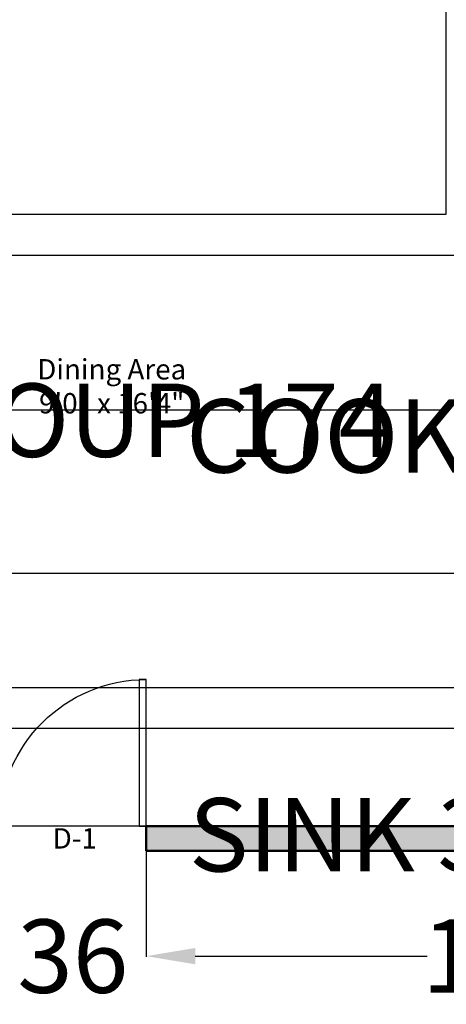
# Model space of a CAD drawing. Units: inches. Extents: x -478 to 256, y -93 to 343.
# Tile 2 of 5: x -211 to -106, y -93 to 149. Entities that reach past the tile are written whole.
import ezdxf

# ---------------------------------------------------------------- set-up
doc = ezdxf.new("R2010")
doc.units = ezdxf.units.IN
for name, color, linetype, lineweight in [('A-ANNO-DIMS', 2, 'Continuous', 18), ('A-ANNO-TEXT', 7, 'Continuous', 18), ('A-AREA-IDEN', 7, 'Continuous', 18), ('A-DOOR', 3, 'Continuous', 25), ('A-WALL-PATT', 8, 'Continuous', 13), ('Outer Wall', 1, 'Continuous', 50)]:
    doc.layers.add(name, color=color, linetype=linetype, lineweight=lineweight)
doc.styles.get("Standard").update_dxf_attribs({"font": 'arial.ttf'})
doc.dimstyles.get("Standard").update_dxf_attribs({"dimtxt": 18, "dimasz": 12, "dimexe": 0.18, "dimexo": 0.0625, "dimgap": 0.09, "dimtad": 0, "dimtih": 1, "dimtoh": 1, "dimdec": 0, "dimzin": 0, "dimdsep": 46, "dimlunit": 3, "dimtxsty": 'Standard', "dimcen": 0.09, "dimadec": 0, "dimazin": 0, "dimtfac": 1, "dimtdec": 0, "dimtofl": 0, "dimtmove": 0, "dimatfit": 3, "dimfxl": 1, "dimtolj": 1, "dimtzin": 0, "dimarcsym": 0})

# ---------------------------------------------------------------- blocks, each defined once
blk = doc.blocks.new('*U14')
for p, q in [((0, 0), (0, -6)), ((36, 0), (36, -6))]:
    blk.add_line(p, q)
blk.add_lwpolyline([(0, 0), (0, 36), (1.75, 36), (1.75, 0)], close=True)
blk.add_arc((0, 0), 36, 0, 90)
blk = doc.blocks.new('*D19')
at = {"layer": 'A-ANNO-DIMS', "color": 0, "lineweight": -2, "transparency": 16777216}
for p, q in [((-8.33, 86.09), (-4.09, 86.09)), ((-4.27, 74.09), (-4.27, 70.61)), ((-8.33, 58.61), (-4.09, 58.61)), ((-4.27, 58.61), (-4.27, 46.61)), ((-4.27, 46.61), (-16.27, 46.61))]:
    blk.add_line(p, q, dxfattribs=at)
at = {"layer": 'A-ANNO-DIMS', "color": 0, "transparency": 16777216}
for points in [[(-6.27, 74.09), (-2.27, 74.09), (-4.27, 86.09)], [(-6.27, 70.61), (-2.27, 70.61), (-4.27, 58.61)]]:
    blk.add_solid(points, dxfattribs=at)
at = {"layer": 'Defpoints', "color": 0, "transparency": 16777216}
for p in [(-8.39, 86.09), (-8.39, 58.61), (-4.27, 58.61)]:
    blk.add_point(p, dxfattribs=at)
at = {"layer": 'A-ANNO-DIMS', "color": 0, "transparency": 16777216, "insert": (-95.51, 46.61), "char_height": 18, "attachment_point": 5}
blk.add_mtext('\\A1;COOKTOP 27', dxfattribs=at)
blk = doc.blocks.new('*D21')
at = {"layer": 'A-ANNO-DIMS', "color": 0, "lineweight": -2, "transparency": 16777216}
for p, q in [((-67.57, -46.21), (-67.57, -51.43)), ((-33.56, -46.21), (-33.56, -51.43)), ((-67.57, -51.25), (-79.57, -51.25)), ((-45.56, -51.25), (-55.57, -51.25))]:
    blk.add_line(p, q, dxfattribs=at)
at = {"layer": 'A-ANNO-DIMS', "color": 0, "transparency": 16777216}
for points in [[(-55.57, -49.25), (-55.57, -53.25), (-67.57, -51.25)], [(-45.56, -49.25), (-45.56, -53.25), (-33.56, -51.25)]]:
    blk.add_solid(points, dxfattribs=at)
at = {"layer": 'Defpoints', "color": 0, "transparency": 16777216}
for p in [(-67.57, -46.15), (-33.56, -46.15), (-67.57, -51.25)]:
    blk.add_point(p, dxfattribs=at)
at = {"layer": 'A-ANNO-DIMS', "color": 0, "transparency": 16777216, "insert": (-125.31, -51.25), "char_height": 18, "attachment_point": 5}
blk.add_mtext('\\A1;SINK 34', dxfattribs=at)
blk = doc.blocks.new('*D25')
at = {"layer": 'A-ANNO-DIMS', "color": 0, "lineweight": -2, "transparency": 16777216}
for p, q in [((-116.04, 214.73), (-116.04, 226.73)), ((-118.49, 202.73), (-115.86, 202.73)), ((-118.49, 185.95), (-115.86, 185.95)), ((-116.04, 173.95), (-116.04, 161.95)), ((-116.04, 161.95), (-128.04, 161.95))]:
    blk.add_line(p, q, dxfattribs=at)
at = {"layer": 'A-ANNO-DIMS', "color": 0, "transparency": 16777216}
for points in [[(-118.04, 214.73), (-114.04, 214.73), (-116.04, 202.73)], [(-118.04, 173.95), (-114.04, 173.95), (-116.04, 185.95)]]:
    blk.add_solid(points, dxfattribs=at)
at = {"layer": 'Defpoints', "color": 0, "transparency": 16777216}
for p in [(-118.56, 202.73), (-118.56, 185.95), (-116.04, 185.95)]:
    blk.add_point(p, dxfattribs=at)
at = {"layer": 'A-ANNO-DIMS', "color": 0, "transparency": 16777216, "insert": (-181.85, 161.95), "char_height": 18, "attachment_point": 5}
blk.add_mtext('\\A1;BASIN 17', dxfattribs=at)
blk = doc.blocks.new('*D29')
at = {"layer": 'A-ANNO-DIMS', "color": 0, "lineweight": -2, "transparency": 16777216}
for p, q in [((-263.32, 137.36), (-237.13, 137.36)), ((-237.31, 125.36), (-237.31, 59.86)), ((-237.31, -24.45), (-237.31, 41.05)), ((-263.32, -36.45), (-237.13, -36.45))]:
    blk.add_line(p, q, dxfattribs=at)
at = {"layer": 'A-ANNO-DIMS', "color": 0, "transparency": 16777216}
for points in [[(-239.31, 125.36), (-235.31, 125.36), (-237.31, 137.36)], [(-239.31, -24.45), (-235.31, -24.45), (-237.31, -36.45)]]:
    blk.add_solid(points, dxfattribs=at)
at = {"layer": 'Defpoints', "color": 0, "transparency": 16777216}
for p in [(-263.38, 137.36), (-263.38, -36.45), (-237.31, -36.45)]:
    blk.add_point(p, dxfattribs=at)
at = {"layer": 'A-ANNO-DIMS', "color": 0, "transparency": 16777216, "insert": (-237.31, 50.46), "char_height": 18, "attachment_point": 5}
blk.add_mtext('\\A1;SEATING GROUP 174', dxfattribs=at)
blk = doc.blocks.new('*D34')
at = {"layer": 'A-ANNO-DIMS', "color": 0, "lineweight": -2, "transparency": 16777216}
for p, q in [((-215.855811, -55.221403), (-215.855811, -81.203903)), ((-179.855811, -55.221403), (-179.855811, -81.203903)), ((-227.855811, -81.023903), (-239.855811, -81.023903)), ((-167.855811, -81.023903), (-155.855811, -81.023903))]:
    blk.add_line(p, q, dxfattribs=at)
at = {"layer": 'A-ANNO-DIMS', "color": 0, "transparency": 16777216}
for points in [[(-227.855811, -79.023903), (-227.855811, -83.023903), (-215.855811, -81.023903)], [(-167.855811, -79.023903), (-167.855811, -83.023903), (-179.855811, -81.023903)]]:
    blk.add_solid(points, dxfattribs=at)
at = {"layer": 'Defpoints', "color": 0, "transparency": 16777216}
for p in [(-215.855811, -55.158903), (-179.855811, -55.158903), (-179.855811, -81.023903)]:
    blk.add_point(p, dxfattribs=at)
at = {"layer": 'A-ANNO-DIMS', "color": 0, "transparency": 16777216, "insert": (-197.855811, -81.023903), "char_height": 18, "attachment_point": 5}
blk.add_mtext('\\A1;36', dxfattribs=at)
blk = doc.blocks.new('*D35')
at = {"layer": 'A-ANNO-DIMS', "color": 0, "lineweight": -2, "transparency": 16777216}
for p, q in [((-3.86, -49.22), (-3.86, -81.2)), ((-179.86, -55.22), (-179.86, -81.2)), ((-167.86, -81.02), (-110.98, -81.02)), ((-15.86, -81.02), (-72.73, -81.02))]:
    blk.add_line(p, q, dxfattribs=at)
at = {"layer": 'A-ANNO-DIMS', "color": 0, "transparency": 16777216}
for points in [[(-167.86, -79.02), (-167.86, -83.02), (-179.86, -81.02)], [(-15.86, -79.02), (-15.86, -83.02), (-3.86, -81.02)]]:
    blk.add_solid(points, dxfattribs=at)
at = {"layer": 'Defpoints', "color": 0, "transparency": 16777216}
for p in [(-3.86, -49.16), (-179.86, -55.16), (-3.86, -81.02)]:
    blk.add_point(p, dxfattribs=at)
at = {"layer": 'A-ANNO-DIMS', "color": 0, "transparency": 16777216, "insert": (-91.86, -81.02), "char_height": 18, "attachment_point": 5}
blk.add_mtext('\\A1;176', dxfattribs=at)
blk = doc.blocks.new('*D52')
at = {"layer": 'A-ANNO-DIMS', "color": 0, "lineweight": -2, "transparency": 16777216}
for p, q in [((-427.72, 12.84), (-427.72, 24.84)), ((-427.72, 24.84), (-415.72, 24.84)), ((0.08, 12.84), (-427.9, 12.84)), ((-427.72, -3.16), (-427.72, 0.84)), ((0.08, -15.16), (-427.9, -15.16))]:
    blk.add_line(p, q, dxfattribs=at)
at = {"layer": 'A-ANNO-DIMS', "color": 0, "transparency": 16777216}
for points in [[(-429.72, 0.84), (-425.72, 0.84), (-427.72, 12.84)], [(-429.72, -3.16), (-425.72, -3.16), (-427.72, -15.16)]]:
    blk.add_solid(points, dxfattribs=at)
at = {"layer": 'Defpoints', "color": 0, "transparency": 16777216}
for p in [(-427.72, 12.84), (0.14, 12.84), (0.14, -15.16)]:
    blk.add_point(p, dxfattribs=at)
at = {"layer": 'A-ANNO-DIMS', "color": 0, "transparency": 16777216, "insert": (-402.57, 24.84), "char_height": 18, "attachment_point": 5}
blk.add_mtext('\\A1;28', dxfattribs=at)
blk = doc.blocks.new('*D53')
at = {"layer": 'A-ANNO-DIMS', "color": 0, "lineweight": -2, "transparency": 16777216}
for p, q in [((-118.28, 330.71), (-130.28, 330.71)), ((-106.28, 101.01), (-106.28, 330.89)), ((-82.28, 101.01), (-82.28, 330.89)), ((-70.28, 330.71), (-58.28, 330.71))]:
    blk.add_line(p, q, dxfattribs=at)
at = {"layer": 'A-ANNO-DIMS', "color": 0, "transparency": 16777216}
for points in [[(-118.28, 332.71), (-118.28, 328.71), (-106.28, 330.71)], [(-70.28, 332.71), (-70.28, 328.71), (-82.28, 330.71)]]:
    blk.add_solid(points, dxfattribs=at)
at = {"layer": 'Defpoints', "color": 0, "transparency": 16777216}
for p in [(-82.28, 330.71), (-106.28, 100.95), (-82.28, 100.95)]:
    blk.add_point(p, dxfattribs=at)
at = {"layer": 'A-ANNO-DIMS', "color": 0, "transparency": 16777216, "insert": (-45.18, 330.71), "char_height": 18, "attachment_point": 5}
blk.add_mtext('\\A1;24', dxfattribs=at)
blk = doc.blocks.new('*D54')
at = {"layer": 'A-ANNO-DIMS', "color": 0, "lineweight": -2, "transparency": 16777216}
for p, q in [((-106.35, 100.95), (-427.9, 100.95)), ((-427.72, 88.95), (-427.72, 86.23)), ((-427.72, 64.95), (-427.72, 67.67)), ((-106.35, 52.95), (-427.9, 52.95))]:
    blk.add_line(p, q, dxfattribs=at)
at = {"layer": 'A-ANNO-DIMS', "color": 0, "transparency": 16777216}
for points in [[(-429.72, 88.95), (-425.72, 88.95), (-427.72, 100.95)], [(-429.72, 64.95), (-425.72, 64.95), (-427.72, 52.95)]]:
    blk.add_solid(points, dxfattribs=at)
at = {"layer": 'Defpoints', "color": 0, "transparency": 16777216}
for p in [(-427.72, 100.95), (-106.28, 100.95), (-106.28, 52.95)]:
    blk.add_point(p, dxfattribs=at)
at = {"layer": 'A-ANNO-DIMS', "color": 0, "transparency": 16777216, "insert": (-427.72, 76.95), "char_height": 18, "attachment_point": 5}
blk.add_mtext('\\A1;48', dxfattribs=at)
blk = doc.blocks.new('*D58')
at = {"layer": 'A-ANNO-DIMS', "color": 0, "lineweight": -2, "transparency": 16777216}
for p, q in [((-427.720811, -13.158903), (-427.720811, -1.158903)), ((-99.918311, -25.158903), (-427.900811, -25.158903)), ((-99.918311, -49.158903), (-427.900811, -49.158903)), ((-427.720811, -61.158903), (-427.720811, -73.158903))]:
    blk.add_line(p, q, dxfattribs=at)
at = {"layer": 'A-ANNO-DIMS', "color": 0, "transparency": 16777216}
for points in [[(-429.720811, -13.158903), (-425.720811, -13.158903), (-427.720811, -25.158903)], [(-429.720811, -61.158903), (-425.720811, -61.158903), (-427.720811, -49.158903)]]:
    blk.add_solid(points, dxfattribs=at)
at = {"layer": 'Defpoints', "color": 0, "transparency": 16777216}
for p in [(-427.720811, -25.158903), (-99.855811, -25.158903), (-99.855811, -49.158903)]:
    blk.add_point(p, dxfattribs=at)
at = {"layer": 'A-ANNO-DIMS', "color": 0, "transparency": 16777216, "insert": (-427.720811, -37.158903), "char_height": 18, "attachment_point": 5}
blk.add_mtext('\\A1;24', dxfattribs=at)
blk = doc.blocks.new('*D61')
at = {"layer": 'A-ANNO-DIMS', "color": 0, "lineweight": -2, "transparency": 16777216}
for p, q in [((-106.35, 52.95), (-427.9, 52.95)), ((-427.72, 40.95), (-427.72, 23.18)), ((-427.72, -13.16), (-427.72, 4.61)), ((-99.92, -25.16), (-427.9, -25.16))]:
    blk.add_line(p, q, dxfattribs=at)
at = {"layer": 'A-ANNO-DIMS', "color": 0, "transparency": 16777216}
for points in [[(-429.72, 40.95), (-425.72, 40.95), (-427.72, 52.95)], [(-429.72, -13.16), (-425.72, -13.16), (-427.72, -25.16)]]:
    blk.add_solid(points, dxfattribs=at)
at = {"layer": 'Defpoints', "color": 0, "transparency": 16777216}
for p in [(-427.72, 52.95), (-106.28, 52.95), (-99.86, -25.16)]:
    blk.add_point(p, dxfattribs=at)
at = {"layer": 'A-ANNO-DIMS', "color": 0, "transparency": 16777216, "insert": (-427.72, 13.9), "char_height": 18, "attachment_point": 5}
blk.add_mtext('\\A1;78.11', dxfattribs=at)
blk = doc.blocks.new('*D66')
at = {"layer": 'A-ANNO-DIMS', "color": 0, "lineweight": -2, "transparency": 16777216}
for p, q in [((24.08, 150.84), (-427.9, 150.84)), ((-427.72, 138.84), (-427.72, 130.12)), ((-427.72, 102.84), (-427.72, 111.56)), ((24.08, 90.84), (-427.9, 90.84))]:
    blk.add_line(p, q, dxfattribs=at)
at = {"layer": 'A-ANNO-DIMS', "color": 0, "transparency": 16777216}
for points in [[(-429.72, 138.84), (-425.72, 138.84), (-427.72, 150.84)], [(-429.72, 102.84), (-425.72, 102.84), (-427.72, 90.84)]]:
    blk.add_solid(points, dxfattribs=at)
at = {"layer": 'Defpoints', "color": 0, "transparency": 16777216}
for p in [(-427.72, 150.84), (24.14, 150.84), (24.14, 90.84)]:
    blk.add_point(p, dxfattribs=at)
at = {"layer": 'A-ANNO-DIMS', "color": 0, "transparency": 16777216, "insert": (-427.72, 120.84), "char_height": 18, "attachment_point": 5}
blk.add_mtext('\\A1;60', dxfattribs=at)
blk = doc.blocks.new('*D68')
at = {"layer": 'A-ANNO-DIMS', "color": 0, "lineweight": -2, "transparency": 16777216}
for p, q in [((-427.720811, -13.158903), (-427.720811, -1.158903)), ((72.081689, -25.158903), (-427.900811, -25.158903)), ((72.081689, -49.158903), (-427.900811, -49.158903)), ((-427.720811, -61.158903), (-427.720811, -73.158903))]:
    blk.add_line(p, q, dxfattribs=at)
at = {"layer": 'A-ANNO-DIMS', "color": 0, "transparency": 16777216}
for points in [[(-429.720811, -13.158903), (-425.720811, -13.158903), (-427.720811, -25.158903)], [(-429.720811, -61.158903), (-425.720811, -61.158903), (-427.720811, -49.158903)]]:
    blk.add_solid(points, dxfattribs=at)
at = {"layer": 'Defpoints', "color": 0, "transparency": 16777216}
for p in [(-427.720811, -25.158903), (72.144189, -25.158903), (72.144189, -49.158903)]:
    blk.add_point(p, dxfattribs=at)
at = {"layer": 'A-ANNO-DIMS', "color": 0, "transparency": 16777216, "insert": (-427.720811, -37.158903), "char_height": 18, "attachment_point": 5}
blk.add_mtext('\\A1;24', dxfattribs=at)

msp = doc.modelspace()

# ---------------------------------------------------------------- hatches: boundary and pattern name
at = {"layer": 'A-WALL-PATT'}
h = msp.add_hatch(color=256, dxfattribs=at)
h.dxf.hatch_style = 1
h.paths.add_polyline_path([(-395.856, 298.841), (72.144, 298.841), (72.144, 20.841), (78.144, 20.841), (78.144, 304.841), (-401.856, 304.841), (-401.856, -55.159), (-215.856, -55.159), (-215.856, -49.159), (-395.856, -49.159)])
h.paths.add_polyline_path([(78.144, -15.159), (72.144, -15.159), (72.144, -49.159), (-179.856, -49.159), (-179.856, -55.159), (78.144, -55.159)], flags=17)

# ---------------------------------------------------------------- linework, layer by layer
at = {"layer": 'Outer Wall'}
for p in [(72.144, -49.159), (-179.856, -55.159)]:
    msp.add_line(p, (-179.856, -49.159), dxfattribs=at)
msp.add_lwpolyline([(78.144, -15.159), (78.144, -55.159), (-179.856, -55.159)], dxfattribs=at)

# ---------------------------------------------------------------- block references
at = {"layer": 'A-DOOR', "xscale": -1}
msp.add_blockref('*U14', (-179.856, -49.159), dxfattribs=at)

# ---------------------------------------------------------------- texts
at = {"layer": 'A-ANNO-TEXT', "insert": (-187.867, -49.623), "char_height": 5, "attachment_point": 3}
msp.add_mtext_dynamic_manual_height_columns('\\pxqc;{\\fTimes New Roman|b0|i0|c0|p18;D-1}', width=19.01487, gutter_width=12.5, heights=[0], dxfattribs=at)
at = {"layer": 'A-AREA-IDEN', "insert": (-169.725, 65.457), "char_height": 5, "attachment_point": 3}
msp.add_mtext_dynamic_manual_height_columns('\\pxqc;{\\fTimes New Roman|b0|i0|c0|p18;Dining Area\\P9\'0" x 16\'4"}', width=37.20338, gutter_width=12.5, heights=[0], dxfattribs=at)

# ---------------------------------------------------------------- dimensions: what is measured, and where the dimension line sits
at = {"layer": 'A-ANNO-DIMS'}
for base, p1, p2, picture, middle in [((-82.284, 330.706), (-106.284, 100.949), (-82.284, 100.949), '*D53', (-45.185, 330.706)), ((-3.856, -81.024), (-179.856, -55.159), (-3.856, -49.159), '*D35', (-91.856, -81.024)), ((-179.856, -81.024), (-215.856, -55.159), (-179.856, -55.159), '*D34', (-197.856, -81.024))]:
    dim = msp.add_linear_dim(base=base, p1=p1, p2=p2, dimstyle='Standard', override={"dimdec": 0, "dimlfac": 1, "dimrnd": 0, "dimzin": 0, "dimdsep": 46, "dimlunit": 2}, dxfattribs=at)
    dim.commit()
    dim.dimension.update_dxf_attribs({"geometry": picture, "text_midpoint": middle})
for base, p1, p2, angle, text, picture, middle in [((-116.039, 185.945), (-118.556, 202.731), (-118.556, 185.945), 270, 'BASIN <>', '*D25', (-181.846, 161.945)), ((-237.313, -36.446), (-263.384, 137.358), (-263.384, -36.446), 270, 'SEATING GROUP <>', '*D29', (-237.313, 50.456)), ((-4.27, 58.61), (-8.392, 86.093), (-8.392, 58.61), 270, 'COOKTOP <>', '*D19', (-95.512, 46.61)), ((-67.568, -51.249), (-33.56, -46.147), (-67.568, -46.147), 180, 'SINK <>', '*D21', (-125.309, -51.249))]:
    dim = msp.add_linear_dim(base=base, p1=p1, p2=p2, angle=angle, text=text, dimstyle='Standard', override={"dimdec": 0, "dimlfac": 1, "dimrnd": 0, "dimzin": 0, "dimdsep": 46, "dimlunit": 2}, dxfattribs=at)
    dim.commit()
    dim.dimension.update_dxf_attribs({"geometry": picture, "text_midpoint": middle})
for base, p1, p2, override, picture, middle in [((-427.721, 150.841), (24.144, 90.841), (24.144, 150.841), {"dimdec": 0, "dimlfac": 1, "dimrnd": 0, "dimzin": 0, "dimdsep": 46, "dimlunit": 2}, '*D66', (-427.721, 120.841)), ((-427.721, 100.949), (-106.284, 52.949), (-106.284, 100.949), {"dimdec": 0, "dimlfac": 1, "dimrnd": 0, "dimzin": 0, "dimdsep": 46, "dimlunit": 2}, '*D54', (-427.721, 76.949)), ((-427.721, 52.949), (-99.856, -25.159), (-106.284, 52.949), {"dimdec": 2, "dimlfac": 1, "dimrnd": 0, "dimzin": 0, "dimdsep": 46, "dimlunit": 2}, '*D61', (-427.721, 13.895)), ((-427.721, 12.841), (0.144, -15.159), (0.144, 12.841), {"dimdec": 0, "dimlfac": 1, "dimrnd": 0, "dimzin": 0, "dimdsep": 46, "dimlunit": 2}, '*D52', (-402.567, 24.841)), ((-427.721, -25.159), (-99.856, -49.159), (-99.856, -25.159), {"dimdec": 0, "dimlfac": 1, "dimrnd": 0, "dimzin": 0, "dimdsep": 46, "dimlunit": 2}, '*D58', (-427.721, -37.159)), ((-427.721, -25.159), (72.144, -49.159), (72.144, -25.159), {"dimdec": 0, "dimlfac": 1, "dimrnd": 0, "dimzin": 0, "dimdsep": 46, "dimlunit": 2}, '*D68', (-427.721, -37.159))]:
    dim = msp.add_linear_dim(base=base, p1=p1, p2=p2, angle=90, dimstyle='Standard', override=override, dxfattribs=at)
    dim.commit()
    dim.dimension.update_dxf_attribs({"geometry": picture, "text_midpoint": middle})

doc.saveas('drawing.dxf')
